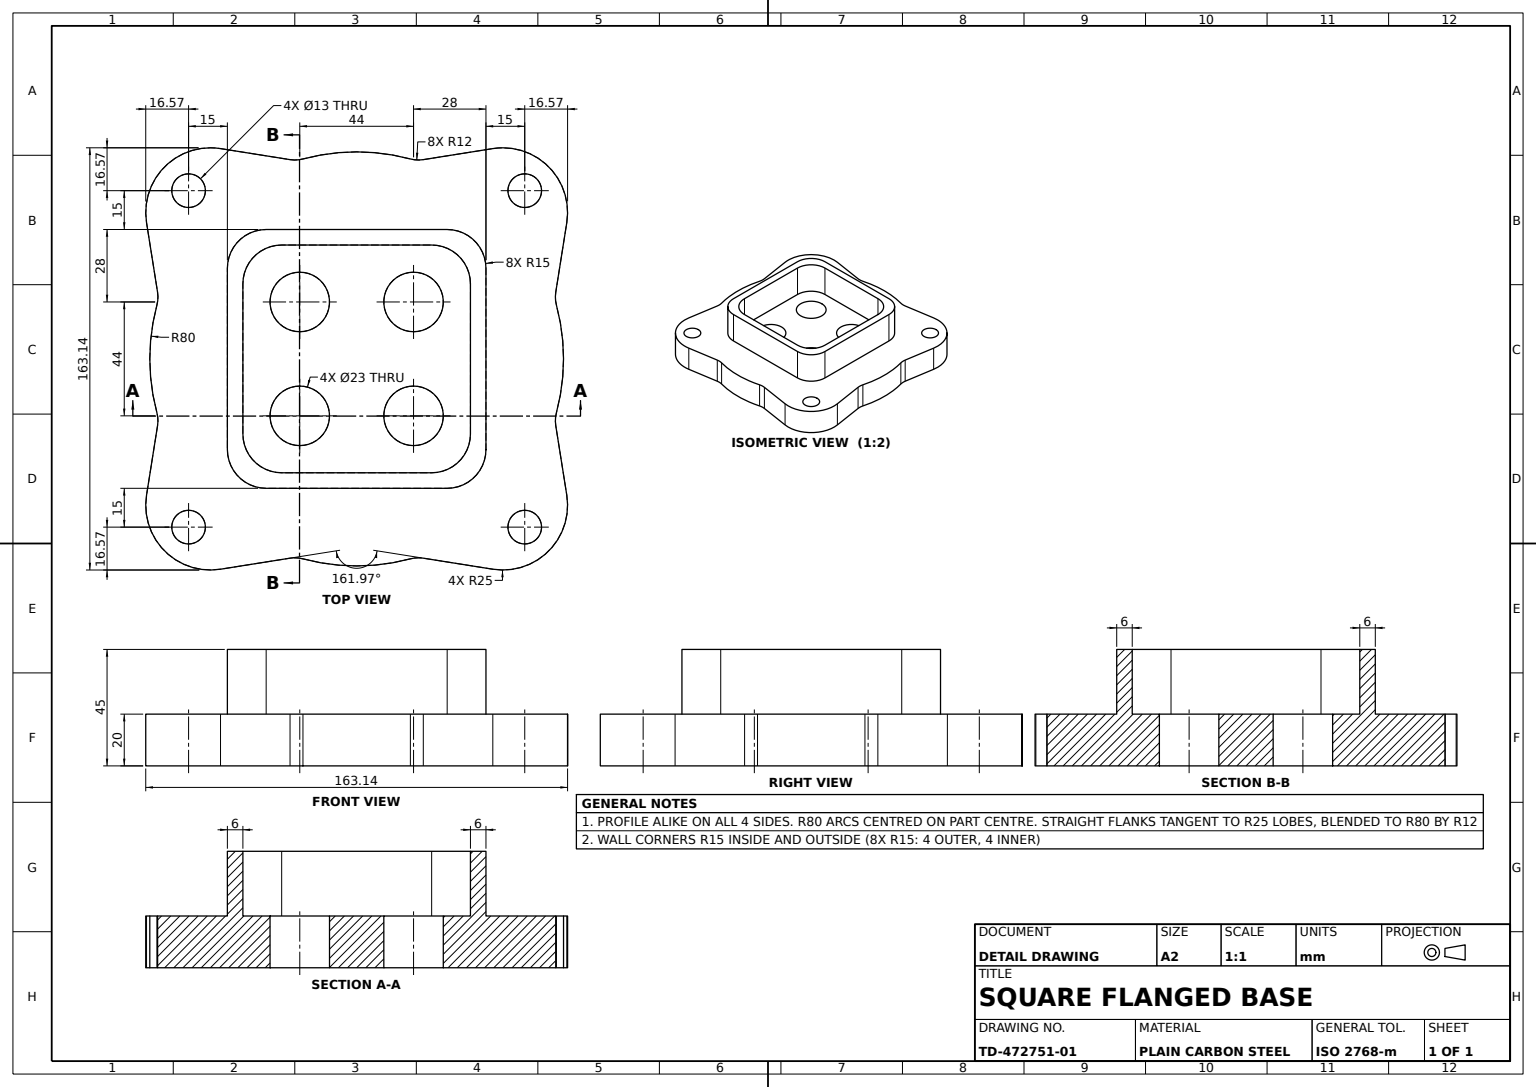
SolidWorks part; units mm, degrees
material "Plain Carbon Steel"
ref_plane "Front Plane" through (0, 0, 0) normal (0, 0, 1) x (1, 0, 0)
ref_plane "Top Plane" through (0, 0, 0) normal (0, 1, 0) x (1, 0, 0)
ref_plane "Right Plane" through (0, 0, 0) normal (1, 0, 0) x (0, 0, -1)
sketch "Lobed Base Profile" plane through (0, 0, 0) normal (0, 1, 0) x (1, 0, 0)
  line L0 (52.6503, -81.2596) -> (23.148, -76.5779)
  line L1 (52.6503, 81.2596) -> (23.148, 76.5779)
  line L2 (81.2596, 52.6503) -> (76.5779, 23.148)
  line L3 (81.2596, -52.6503) -> (76.5779, -23.148)
  line L4 (-81.2596, -52.6503) -> (-76.5779, -23.148)
  line L5 (-52.6503, -81.2596) -> (-23.148, -76.5779)
  line L6 (-52.6503, 81.2596) -> (-23.148, 76.5779)
  line L7 (-81.2596, 52.6503) -> (-76.5779, 23.148)
  arc A0 (23.148, 76.5779) -> (-23.148, 76.5779) centre (0, 0) ccw
  arc A3 (81.2596, 52.6503) -> (52.6503, 81.2596) centre (56.5685, 56.5685) ccw
  arc A4 (52.6503, -81.2596) -> (81.2596, -52.6503) centre (56.5685, -56.5685) ccw
  arc A5 (-81.2596, -52.6503) -> (-52.6503, -81.2596) centre (-56.5685, -56.5685) ccw
  arc A6 (-52.6503, 81.2596) -> (-81.2596, 52.6503) centre (-56.5685, 56.5685) ccw
  arc A7 (76.5779, -23.148) -> (76.5779, 23.148) centre (0, 0) ccw
  arc A8 (-23.148, -76.5779) -> (23.148, -76.5779) centre (0, 0) ccw
  arc A9 (-76.5779, 23.148) -> (-76.5779, -23.148) centre (0, 0) ccw
  dimension "D1" = 160
  dimension "D2" = 4
  dimension "D3" = 25
  dimension "D4" = 25
  dimension "D5" = 56.5685
  dimension "D6" = 29.5024
  dimension "D7" = 29.5024
  dimension "D8" = 72.0036
extrude "Lobed Base Plate" add sketch "Lobed Base Profile" along normal blind 20
sketch "Square Wall Profile" plane through (0, 20, 0) normal (0, 1, 0) x (1, 0, 0)
  line L0 (44, -1.6416) -> (44, -29)
  line L1 (29, -44) -> (-29, -44)
  line L2 (50, -1.6416) -> (50, -35)
  line L3 (35, -50) -> (-35, -50)
  line L4 (-50, -35) -> (-50, 35)
  line L5 (-35, 50) -> (35, 50)
  line L6 (50, 35) -> (50, -1.6416)
  line L7 (-44, -29) -> (-44, 29)
  line L8 (-29, 44) -> (29, 44)
  line L9 (44, 29) -> (44, -1.6416)
  line L10 (-50, -50) -> (-50, 50) construction
  line L11 (-50, 50) -> (50, 50) construction
  line L12 (50, -50) -> (-50, -50) construction
  line L13 (50, -1.6416) -> (50, -50) construction
  line L14 (50, 50) -> (50, -1.6416) construction
  line L15 (-44, 44) -> (44, 44) construction
  line L16 (-44, -44) -> (-44, 44) construction
  line L17 (44, -44) -> (-44, -44) construction
  line L18 (44, -1.6416) -> (44, -44) construction
  line L19 (44, 44) -> (44, -1.6416) construction
  arc A0 (-50, 35) -> (-35, 50) centre (-35, 35) cw
  arc A1 (-35, -50) -> (-50, -35) centre (-35, -35) cw
  arc A2 (50, -35) -> (35, -50) centre (35, -35) cw
  arc A3 (35, 50) -> (50, 35) centre (35, 35) cw
  arc A4 (-29, 44) -> (-44, 29) centre (-29, 29) ccw
  arc A5 (-29, -44) -> (-44, -29) centre (-29, -29) cw
  arc A6 (44, -29) -> (29, -44) centre (29, -29) cw
  arc A7 (29, 44) -> (44, 29) centre (29, 29) cw
  point P15 (-50, 50)
  dimension "D6" = 15
  dimension "D2" = 15
  dimension "D3" = 29
  dimension "D1" = 6
  dimension "D4" = 50
  dimension "D5" = 50
  dimension "D7" = 35
  dimension "D8" = 1.6416
extrude "Square Pocket Wall" add sketch "Square Wall Profile" along normal blind 25
sketch "Pocket Holes Sketch" plane through (0, 20, 0) normal (0, 1, 0) x (1, 0, 0)
  circle A0 centre (22, -22) radius 11.5
  circle A1 centre (22, 22) radius 11.5
  circle A2 centre (-22, 22) radius 11.5
  circle A3 centre (-22, -22) radius 11.5
  dimension "D1" = 23
  dimension "D2" = 23
  dimension "D3" = 23
  dimension "D4" = 23
  dimension "D5" = 22
  dimension "D6" = 22
  dimension "D7" = 22
  dimension "D8" = 22
  dimension "D9" = 22
  dimension "D10" = 22
  dimension "D11" = 22
  dimension "D12" = 22
extrude "Pocket Floor Holes 4x" cut sketch "Pocket Holes Sketch" against normal blind 25
fillet "Edge Fillet R12 A" radius 12 1 edges at (23.148, 10, 76.5779)
fillet "Edge Fillet R12 B" radius 12 1 edges at (-23.148, 10, 76.5779)
fillet "Edge Fillet R12 C" radius 12 1 edges at (23.148, 10, -76.5779)
fillet "Edge Fillet R12 D" radius 12 1 edges at (-23.148, 10, -76.5779)
fillet "Edge Fillet R12 E" radius 12 1 edges at (76.5779, 10, -23.148)
fillet "Edge Fillet R12 F" radius 12 1 edges at (76.5779, 10, 23.148)
fillet "Edge Fillet R12 G" radius 12 1 edges at (-76.5779, 10, 23.148)
fillet "Edge Fillet R12 H" radius 12 1 edges at (-76.5779, 10, -23.148)
sketch "Mounting Holes Sketch" plane through (0, 20, 0) normal (0, 1, 0) x (1, 0, 0)
  circle A0 centre (65, 65) radius 6.5
  circle A1 centre (65, -65) radius 6.5
  circle A2 centre (-65, -65) radius 6.5
  circle A3 centre (-65, 65) radius 6.5
  dimension "D1" = 13
  dimension "D2" = 13
  dimension "D3" = 13
  dimension "D4" = 13
  dimension "D5" = 65
  dimension "D6" = 65
  dimension "D7" = 65
  dimension "D8" = 65
  dimension "D9" = 65
  dimension "D10" = 65
  dimension "D11" = 65
  dimension "D12" = 65
extrude "Mounting Holes 4x" cut sketch "Mounting Holes Sketch" against normal blind 25
